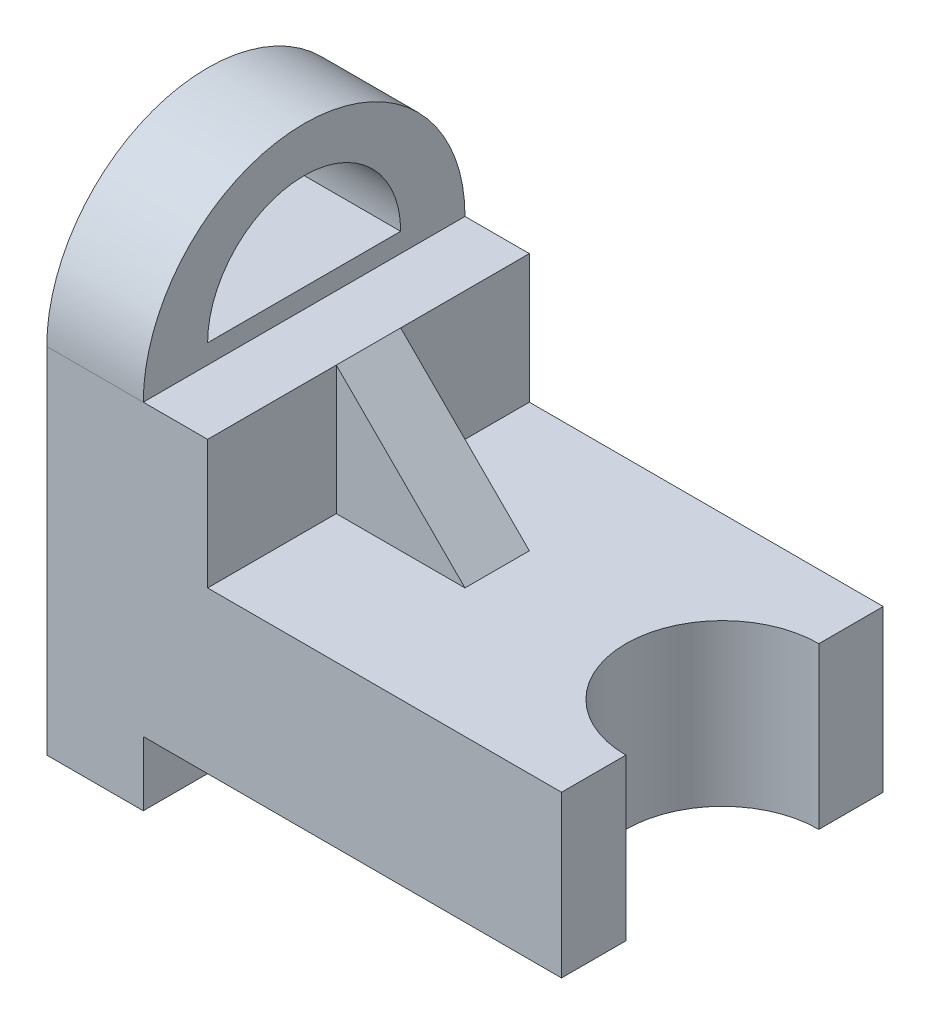
ISO-10303-21;
HEADER;
FILE_DESCRIPTION(('STEP AP214'),'2;1');
FILE_NAME('part.step','',(''),(''),'','','');
FILE_SCHEMA(('AUTOMOTIVE_DESIGN { 1 0 10303 214 1 1 1 1 }'));
ENDSEC;
DATA;
#1=APPLICATION_CONTEXT('core data for automotive mechanical design processes');
#2=APPLICATION_PROTOCOL_DEFINITION('international standard','automotive_design',2000,#1);
#3=PRODUCT_CONTEXT('',#1,'mechanical');
#4=PRODUCT('Part','Part','',(#3));
#5=PRODUCT_RELATED_PRODUCT_CATEGORY('part','',(#4));
#6=PRODUCT_DEFINITION_FORMATION('','',#4);
#7=PRODUCT_DEFINITION_CONTEXT('part definition',#1,'design');
#8=PRODUCT_DEFINITION('design','',#6,#7);
#9=PRODUCT_DEFINITION_SHAPE('','',#8);
#10=(LENGTH_UNIT() NAMED_UNIT(*) SI_UNIT(.MILLI.,.METRE.));
#11=(NAMED_UNIT(*) PLANE_ANGLE_UNIT() SI_UNIT($,.RADIAN.));
#12=(NAMED_UNIT(*) SI_UNIT($,.STERADIAN.) SOLID_ANGLE_UNIT());
#13=UNCERTAINTY_MEASURE_WITH_UNIT(LENGTH_MEASURE(1.E-05),#10,'distance_accuracy_value','');
#14=(GEOMETRIC_REPRESENTATION_CONTEXT(3) GLOBAL_UNCERTAINTY_ASSIGNED_CONTEXT((#13)) GLOBAL_UNIT_ASSIGNED_CONTEXT((#10,
#11,#12)) REPRESENTATION_CONTEXT('',''));
#15=CARTESIAN_POINT('',(0.,0.,0.));
#16=DIRECTION('',(0.,0.,1.));
#17=DIRECTION('',(1.,0.,0.));
#18=AXIS2_PLACEMENT_3D('',#15,#16,#17);
#19=CARTESIAN_POINT('',(40.,35.,20.));
#20=DIRECTION('',(0.707106781186547,0.707106781186548,0.));
#21=DIRECTION('',(-0.707106781186548,0.707106781186547,0.));
#22=AXIS2_PLACEMENT_3D('',#19,#20,#21);
#23=PLANE('',#22);
#24=DIRECTION('',(0.,0.,1.));
#25=VECTOR('',#24,1.);
#26=CARTESIAN_POINT('',(20.,55.,20.));
#27=LINE('',#26,#25);
#28=CARTESIAN_POINT('',(20.,55.,20.));
#29=VERTEX_POINT('',#28);
#30=CARTESIAN_POINT('',(20.,55.,30.));
#31=VERTEX_POINT('',#30);
#32=EDGE_CURVE('E179',#29,#31,#27,.T.);
#33=ORIENTED_EDGE('',*,*,#32,.T.);
#34=DIRECTION('',(-0.707106781186548,0.707106781186547,0.));
#35=VECTOR('',#34,1.);
#36=CARTESIAN_POINT('',(40.,35.,30.));
#37=LINE('',#36,#35);
#38=CARTESIAN_POINT('',(40.,35.,30.));
#39=VERTEX_POINT('',#38);
#40=EDGE_CURVE('E166',#39,#31,#37,.T.);
#41=ORIENTED_EDGE('',*,*,#40,.F.);
#42=DIRECTION('',(0.,0.,1.));
#43=VECTOR('',#42,1.);
#44=CARTESIAN_POINT('',(40.,35.,20.));
#45=LINE('',#44,#43);
#46=CARTESIAN_POINT('',(40.,35.,20.));
#47=VERTEX_POINT('',#46);
#48=EDGE_CURVE('E189',#47,#39,#45,.T.);
#49=ORIENTED_EDGE('',*,*,#48,.F.);
#50=DIRECTION('',(-0.707106781186548,0.707106781186547,0.));
#51=VECTOR('',#50,1.);
#52=CARTESIAN_POINT('',(40.,35.,20.));
#53=LINE('',#52,#51);
#54=EDGE_CURVE('E190',#47,#29,#53,.T.);
#55=ORIENTED_EDGE('',*,*,#54,.T.);
#56=EDGE_LOOP('',(#33,#41,#49,#55));
#57=FACE_BOUND('',#56,.T.);
#58=ADVANCED_FACE('F44',(#57),#23,.T.);
#59=CARTESIAN_POINT('',(20.,0.,0.));
#60=DIRECTION('',(-1.,0.,0.));
#61=DIRECTION('',(0.,0.,1.));
#62=AXIS2_PLACEMENT_3D('',#59,#60,#61);
#63=PLANE('',#62);
#64=DIRECTION('',(0.,-1.,0.));
#65=VECTOR('',#64,1.);
#66=CARTESIAN_POINT('',(20.,55.,20.));
#67=LINE('',#66,#65);
#68=CARTESIAN_POINT('',(20.,35.,20.));
#69=VERTEX_POINT('',#68);
#70=EDGE_CURVE('E195',#29,#69,#67,.T.);
#71=ORIENTED_EDGE('',*,*,#70,.T.);
#72=DIRECTION('',(0.,0.,-1.));
#73=VECTOR('',#72,1.);
#74=CARTESIAN_POINT('',(20.,35.,0.));
#75=LINE('',#74,#73);
#76=CARTESIAN_POINT('',(20.,35.,0.));
#77=VERTEX_POINT('',#76);
#78=EDGE_CURVE('E222',#69,#77,#75,.T.);
#79=ORIENTED_EDGE('',*,*,#78,.T.);
#80=DIRECTION('',(0.,1.,0.));
#81=VECTOR('',#80,1.);
#82=CARTESIAN_POINT('',(20.,55.,0.));
#83=LINE('',#82,#81);
#84=CARTESIAN_POINT('',(20.,55.,0.));
#85=VERTEX_POINT('',#84);
#86=EDGE_CURVE('E225',#77,#85,#83,.T.);
#87=ORIENTED_EDGE('',*,*,#86,.T.);
#88=DIRECTION('',(0.,0.,1.));
#89=VECTOR('',#88,1.);
#90=CARTESIAN_POINT('',(20.,55.,50.));
#91=LINE('',#90,#89);
#92=EDGE_CURVE('E223',#85,#29,#91,.T.);
#93=ORIENTED_EDGE('',*,*,#92,.T.);
#94=EDGE_LOOP('',(#71,#79,#87,#93));
#95=FACE_BOUND('',#94,.T.);
#96=ADVANCED_FACE('F328',(#95),#63,.F.);
#97=CARTESIAN_POINT('',(75.,35.,50.));
#98=DIRECTION('',(-1.,0.,0.));
#99=DIRECTION('',(0.,0.,1.));
#100=AXIS2_PLACEMENT_3D('',#97,#98,#99);
#101=PLANE('',#100);
#102=DIRECTION('',(0.,0.,-1.));
#103=VECTOR('',#102,1.);
#104=CARTESIAN_POINT('',(75.,10.,50.));
#105=LINE('',#104,#103);
#106=CARTESIAN_POINT('',(75.,10.,50.));
#107=VERTEX_POINT('',#106);
#108=CARTESIAN_POINT('',(75.,10.,40.));
#109=VERTEX_POINT('',#108);
#110=EDGE_CURVE('E278',#107,#109,#105,.T.);
#111=ORIENTED_EDGE('',*,*,#110,.T.);
#112=DIRECTION('',(0.,1.,0.));
#113=VECTOR('',#112,1.);
#114=CARTESIAN_POINT('',(75.,10.,40.));
#115=LINE('',#114,#113);
#116=CARTESIAN_POINT('',(75.,35.,40.));
#117=VERTEX_POINT('',#116);
#118=EDGE_CURVE('E196',#109,#117,#115,.T.);
#119=ORIENTED_EDGE('',*,*,#118,.T.);
#120=DIRECTION('',(0.,0.,-1.));
#121=VECTOR('',#120,1.);
#122=CARTESIAN_POINT('',(75.,35.,50.));
#123=LINE('',#122,#121);
#124=CARTESIAN_POINT('',(75.,35.,50.));
#125=VERTEX_POINT('',#124);
#126=EDGE_CURVE('E277',#125,#117,#123,.T.);
#127=ORIENTED_EDGE('',*,*,#126,.F.);
#128=DIRECTION('',(0.,1.,0.));
#129=VECTOR('',#128,1.);
#130=CARTESIAN_POINT('',(75.,35.,50.));
#131=LINE('',#130,#129);
#132=EDGE_CURVE('E251',#107,#125,#131,.T.);
#133=ORIENTED_EDGE('',*,*,#132,.F.);
#134=EDGE_LOOP('',(#111,#119,#127,#133));
#135=FACE_BOUND('',#134,.T.);
#136=ADVANCED_FACE('F304',(#135),#101,.F.);
#137=CARTESIAN_POINT('',(10.,35.,50.));
#138=DIRECTION('',(0.,-1.,0.));
#139=DIRECTION('',(0.,0.,-1.));
#140=AXIS2_PLACEMENT_3D('',#137,#138,#139);
#141=PLANE('',#140);
#142=DIRECTION('',(1.,0.,0.));
#143=VECTOR('',#142,1.);
#144=CARTESIAN_POINT('',(20.,35.,20.));
#145=LINE('',#144,#143);
#146=EDGE_CURVE('E66',#69,#47,#145,.T.);
#147=ORIENTED_EDGE('',*,*,#146,.T.);
#148=ORIENTED_EDGE('',*,*,#48,.T.);
#149=DIRECTION('',(1.,0.,0.));
#150=VECTOR('',#149,1.);
#151=CARTESIAN_POINT('',(20.,35.,30.));
#152=LINE('',#151,#150);
#153=CARTESIAN_POINT('',(20.,35.,30.));
#154=VERTEX_POINT('',#153);
#155=EDGE_CURVE('E58',#154,#39,#152,.T.);
#156=ORIENTED_EDGE('',*,*,#155,.F.);
#157=DIRECTION('',(0.,0.,1.));
#158=VECTOR('',#157,1.);
#159=CARTESIAN_POINT('',(20.,35.,30.));
#160=LINE('',#159,#158);
#161=CARTESIAN_POINT('',(20.,35.,50.));
#162=VERTEX_POINT('',#161);
#163=EDGE_CURVE('E170',#154,#162,#160,.T.);
#164=ORIENTED_EDGE('',*,*,#163,.T.);
#165=DIRECTION('',(-1.,0.,0.));
#166=VECTOR('',#165,1.);
#167=CARTESIAN_POINT('',(10.,35.,50.));
#168=LINE('',#167,#166);
#169=EDGE_CURVE('E257',#125,#162,#168,.T.);
#170=ORIENTED_EDGE('',*,*,#169,.F.);
#171=ORIENTED_EDGE('',*,*,#126,.T.);
#172=CARTESIAN_POINT('',(75.,35.,25.));
#173=DIRECTION('',(0.,1.,0.));
#174=DIRECTION('',(0.,0.,1.));
#175=AXIS2_PLACEMENT_3D('',#172,#173,#174);
#176=CIRCLE('',#175,15.);
#177=CARTESIAN_POINT('',(75.,35.,9.99999999999999));
#178=VERTEX_POINT('',#177);
#179=EDGE_CURVE('E188',#178,#117,#176,.T.);
#180=ORIENTED_EDGE('',*,*,#179,.F.);
#181=CARTESIAN_POINT('',(75.,35.,0.));
#182=VERTEX_POINT('',#181);
#183=EDGE_CURVE('E263',#178,#182,#123,.T.);
#184=ORIENTED_EDGE('',*,*,#183,.T.);
#185=DIRECTION('',(-1.,0.,0.));
#186=VECTOR('',#185,1.);
#187=CARTESIAN_POINT('',(10.,35.,0.));
#188=LINE('',#187,#186);
#189=EDGE_CURVE('E272',#182,#77,#188,.T.);
#190=ORIENTED_EDGE('',*,*,#189,.T.);
#191=ORIENTED_EDGE('',*,*,#78,.F.);
#192=EDGE_LOOP('',(#147,#148,#156,#164,#170,#171,#180,#184,#190,#191));
#193=FACE_BOUND('',#192,.T.);
#194=ADVANCED_FACE('F326',(#193),#141,.F.);
#195=CARTESIAN_POINT('',(10.,55.,50.));
#196=DIRECTION('',(-1.,0.,0.));
#197=DIRECTION('',(0.,0.,1.));
#198=AXIS2_PLACEMENT_3D('',#195,#196,#197);
#199=PLANE('',#198);
#200=CARTESIAN_POINT('',(10.,58.,25.));
#201=DIRECTION('',(1.,0.,0.));
#202=DIRECTION('',(0.,0.,-1.));
#203=AXIS2_PLACEMENT_3D('',#200,#201,#202);
#204=CIRCLE('',#203,15.);
#205=CARTESIAN_POINT('',(10.,58.,10.));
#206=VERTEX_POINT('',#205);
#207=CARTESIAN_POINT('',(10.,58.,40.));
#208=VERTEX_POINT('',#207);
#209=EDGE_CURVE('E209',#206,#208,#204,.T.);
#210=ORIENTED_EDGE('',*,*,#209,.F.);
#211=DIRECTION('',(0.,0.,-1.));
#212=VECTOR('',#211,1.);
#213=CARTESIAN_POINT('',(10.,58.,0.));
#214=LINE('',#213,#212);
#215=EDGE_CURVE('E204',#208,#206,#214,.T.);
#216=ORIENTED_EDGE('',*,*,#215,.F.);
#217=EDGE_LOOP('',(#210,#216));
#218=FACE_BOUND('',#217,.T.);
#219=DIRECTION('',(0.,0.,1.));
#220=VECTOR('',#219,1.);
#221=CARTESIAN_POINT('',(10.,55.,50.));
#222=LINE('',#221,#220);
#223=CARTESIAN_POINT('',(10.,55.,0.));
#224=VERTEX_POINT('',#223);
#225=CARTESIAN_POINT('',(10.,55.,50.));
#226=VERTEX_POINT('',#225);
#227=EDGE_CURVE('E216',#224,#226,#222,.T.);
#228=ORIENTED_EDGE('',*,*,#227,.F.);
#229=CARTESIAN_POINT('',(10.,55.,25.));
#230=DIRECTION('',(-1.,0.,0.));
#231=DIRECTION('',(0.,0.,1.));
#232=AXIS2_PLACEMENT_3D('',#229,#230,#231);
#233=CIRCLE('',#232,25.);
#234=EDGE_CURVE('E231',#226,#224,#233,.T.);
#235=ORIENTED_EDGE('',*,*,#234,.F.);
#236=EDGE_LOOP('',(#228,#235));
#237=FACE_BOUND('',#236,.T.);
#238=ADVANCED_FACE('F321',(#218,#237),#199,.F.);
#239=CARTESIAN_POINT('',(10.,0.,50.));
#240=DIRECTION('',(0.,1.,0.));
#241=DIRECTION('',(0.,0.,1.));
#242=AXIS2_PLACEMENT_3D('',#239,#240,#241);
#243=PLANE('',#242);
#244=DIRECTION('',(1.,0.,0.));
#245=VECTOR('',#244,1.);
#246=CARTESIAN_POINT('',(10.,0.,50.));
#247=LINE('',#246,#245);
#248=CARTESIAN_POINT('',(-5.,0.,50.));
#249=VERTEX_POINT('',#248);
#250=CARTESIAN_POINT('',(10.,0.,50.));
#251=VERTEX_POINT('',#250);
#252=EDGE_CURVE('E250',#249,#251,#247,.T.);
#253=ORIENTED_EDGE('',*,*,#252,.F.);
#254=DIRECTION('',(0.,0.,1.));
#255=VECTOR('',#254,1.);
#256=CARTESIAN_POINT('',(-5.,0.,50.));
#257=LINE('',#256,#255);
#258=CARTESIAN_POINT('',(-5.,0.,0.));
#259=VERTEX_POINT('',#258);
#260=EDGE_CURVE('E239',#259,#249,#257,.T.);
#261=ORIENTED_EDGE('',*,*,#260,.F.);
#262=DIRECTION('',(1.,0.,0.));
#263=VECTOR('',#262,1.);
#264=CARTESIAN_POINT('',(10.,0.,0.));
#265=LINE('',#264,#263);
#266=CARTESIAN_POINT('',(10.,0.,0.));
#267=VERTEX_POINT('',#266);
#268=EDGE_CURVE('E246',#259,#267,#265,.T.);
#269=ORIENTED_EDGE('',*,*,#268,.T.);
#270=DIRECTION('',(0.,0.,-1.));
#271=VECTOR('',#270,1.);
#272=CARTESIAN_POINT('',(10.,0.,50.));
#273=LINE('',#272,#271);
#274=EDGE_CURVE('E11',#251,#267,#273,.T.);
#275=ORIENTED_EDGE('',*,*,#274,.F.);
#276=EDGE_LOOP('',(#253,#261,#269,#275));
#277=FACE_BOUND('',#276,.T.);
#278=ADVANCED_FACE('F50',(#277),#243,.F.);
#279=CARTESIAN_POINT('',(10.,10.,50.));
#280=DIRECTION('',(-1.,0.,0.));
#281=DIRECTION('',(0.,0.,1.));
#282=AXIS2_PLACEMENT_3D('',#279,#280,#281);
#283=PLANE('',#282);
#284=DIRECTION('',(0.,1.,0.));
#285=VECTOR('',#284,1.);
#286=CARTESIAN_POINT('',(10.,10.,0.));
#287=LINE('',#286,#285);
#288=CARTESIAN_POINT('',(10.,10.,0.));
#289=VERTEX_POINT('',#288);
#290=EDGE_CURVE('E261',#267,#289,#287,.T.);
#291=ORIENTED_EDGE('',*,*,#290,.T.);
#292=DIRECTION('',(0.,0.,-1.));
#293=VECTOR('',#292,1.);
#294=CARTESIAN_POINT('',(10.,10.,50.));
#295=LINE('',#294,#293);
#296=CARTESIAN_POINT('',(10.,10.,50.));
#297=VERTEX_POINT('',#296);
#298=EDGE_CURVE('E52',#297,#289,#295,.T.);
#299=ORIENTED_EDGE('',*,*,#298,.F.);
#300=DIRECTION('',(0.,1.,0.));
#301=VECTOR('',#300,1.);
#302=CARTESIAN_POINT('',(10.,10.,50.));
#303=LINE('',#302,#301);
#304=EDGE_CURVE('E248',#251,#297,#303,.T.);
#305=ORIENTED_EDGE('',*,*,#304,.F.);
#306=ORIENTED_EDGE('',*,*,#274,.T.);
#307=EDGE_LOOP('',(#291,#299,#305,#306));
#308=FACE_BOUND('',#307,.T.);
#309=ADVANCED_FACE('F315',(#308),#283,.F.);
#310=CARTESIAN_POINT('',(75.,10.,50.));
#311=DIRECTION('',(0.,1.,0.));
#312=DIRECTION('',(0.,0.,1.));
#313=AXIS2_PLACEMENT_3D('',#310,#311,#312);
#314=PLANE('',#313);
#315=CARTESIAN_POINT('',(75.,10.,9.99999999999999));
#316=VERTEX_POINT('',#315);
#317=CARTESIAN_POINT('',(75.,10.,0.));
#318=VERTEX_POINT('',#317);
#319=EDGE_CURVE('E276',#316,#318,#105,.T.);
#320=ORIENTED_EDGE('',*,*,#319,.F.);
#321=CARTESIAN_POINT('',(75.,10.,25.));
#322=DIRECTION('',(0.,1.,0.));
#323=DIRECTION('',(0.,0.,1.));
#324=AXIS2_PLACEMENT_3D('',#321,#322,#323);
#325=CIRCLE('',#324,15.);
#326=EDGE_CURVE('E193',#316,#109,#325,.T.);
#327=ORIENTED_EDGE('',*,*,#326,.T.);
#328=ORIENTED_EDGE('',*,*,#110,.F.);
#329=DIRECTION('',(1.,0.,0.));
#330=VECTOR('',#329,1.);
#331=CARTESIAN_POINT('',(75.,10.,50.));
#332=LINE('',#331,#330);
#333=EDGE_CURVE('E255',#297,#107,#332,.T.);
#334=ORIENTED_EDGE('',*,*,#333,.F.);
#335=ORIENTED_EDGE('',*,*,#298,.T.);
#336=DIRECTION('',(1.,0.,0.));
#337=VECTOR('',#336,1.);
#338=CARTESIAN_POINT('',(75.,10.,0.));
#339=LINE('',#338,#337);
#340=EDGE_CURVE('E262',#289,#318,#339,.T.);
#341=ORIENTED_EDGE('',*,*,#340,.T.);
#342=EDGE_LOOP('',(#320,#327,#328,#334,#335,#341));
#343=FACE_BOUND('',#342,.T.);
#344=ADVANCED_FACE('F290',(#343),#314,.F.);
#345=ORIENTED_EDGE('',*,*,#183,.F.);
#346=DIRECTION('',(0.,1.,0.));
#347=VECTOR('',#346,1.);
#348=CARTESIAN_POINT('',(75.,10.,9.99999999999999));
#349=LINE('',#348,#347);
#350=EDGE_CURVE('E197',#316,#178,#349,.T.);
#351=ORIENTED_EDGE('',*,*,#350,.F.);
#352=ORIENTED_EDGE('',*,*,#319,.T.);
#353=DIRECTION('',(0.,1.,0.));
#354=VECTOR('',#353,1.);
#355=CARTESIAN_POINT('',(75.,35.,0.));
#356=LINE('',#355,#354);
#357=EDGE_CURVE('E270',#318,#182,#356,.T.);
#358=ORIENTED_EDGE('',*,*,#357,.T.);
#359=EDGE_LOOP('',(#345,#351,#352,#358));
#360=FACE_BOUND('',#359,.T.);
#361=ADVANCED_FACE('F297',(#360),#101,.F.);
#362=CARTESIAN_POINT('',(0.,0.,50.));
#363=DIRECTION('',(0.,0.,-1.));
#364=DIRECTION('',(-1.,0.,0.));
#365=AXIS2_PLACEMENT_3D('',#362,#363,#364);
#366=PLANE('',#365);
#367=ORIENTED_EDGE('',*,*,#169,.T.);
#368=DIRECTION('',(0.,-1.,0.));
#369=VECTOR('',#368,1.);
#370=CARTESIAN_POINT('',(20.,55.,50.));
#371=LINE('',#370,#369);
#372=CARTESIAN_POINT('',(20.,55.,50.));
#373=VERTEX_POINT('',#372);
#374=EDGE_CURVE('E173',#373,#162,#371,.T.);
#375=ORIENTED_EDGE('',*,*,#374,.F.);
#376=DIRECTION('',(-1.,0.,0.));
#377=VECTOR('',#376,1.);
#378=CARTESIAN_POINT('',(20.,55.,50.));
#379=LINE('',#378,#377);
#380=EDGE_CURVE('E182',#373,#226,#379,.T.);
#381=ORIENTED_EDGE('',*,*,#380,.T.);
#382=DIRECTION('',(-1.,0.,0.));
#383=VECTOR('',#382,1.);
#384=CARTESIAN_POINT('',(0.,55.,50.));
#385=LINE('',#384,#383);
#386=CARTESIAN_POINT('',(-5.,55.,50.));
#387=VERTEX_POINT('',#386);
#388=EDGE_CURVE('E259',#226,#387,#385,.T.);
#389=ORIENTED_EDGE('',*,*,#388,.T.);
#390=DIRECTION('',(0.,1.,0.));
#391=VECTOR('',#390,1.);
#392=CARTESIAN_POINT('',(-5.,55.,50.));
#393=LINE('',#392,#391);
#394=EDGE_CURVE('E243',#249,#387,#393,.T.);
#395=ORIENTED_EDGE('',*,*,#394,.F.);
#396=ORIENTED_EDGE('',*,*,#252,.T.);
#397=ORIENTED_EDGE('',*,*,#304,.T.);
#398=ORIENTED_EDGE('',*,*,#333,.T.);
#399=ORIENTED_EDGE('',*,*,#132,.T.);
#400=EDGE_LOOP('',(#367,#375,#381,#389,#395,#396,#397,#398,#399));
#401=FACE_BOUND('',#400,.T.);
#402=ADVANCED_FACE('F307',(#401),#366,.F.);
#403=CARTESIAN_POINT('',(0.,0.,0.));
#404=DIRECTION('',(0.,0.,-1.));
#405=DIRECTION('',(-1.,0.,0.));
#406=AXIS2_PLACEMENT_3D('',#403,#404,#405);
#407=PLANE('',#406);
#408=ORIENTED_EDGE('',*,*,#268,.F.);
#409=DIRECTION('',(0.,-1.,0.));
#410=VECTOR('',#409,1.);
#411=CARTESIAN_POINT('',(-5.,0.,0.));
#412=LINE('',#411,#410);
#413=CARTESIAN_POINT('',(-5.,55.,0.));
#414=VERTEX_POINT('',#413);
#415=EDGE_CURVE('E236',#414,#259,#412,.T.);
#416=ORIENTED_EDGE('',*,*,#415,.F.);
#417=DIRECTION('',(-1.,0.,0.));
#418=VECTOR('',#417,1.);
#419=CARTESIAN_POINT('',(0.,55.,0.));
#420=LINE('',#419,#418);
#421=EDGE_CURVE('E249',#224,#414,#420,.T.);
#422=ORIENTED_EDGE('',*,*,#421,.F.);
#423=DIRECTION('',(-1.,0.,0.));
#424=VECTOR('',#423,1.);
#425=CARTESIAN_POINT('',(20.,55.,0.));
#426=LINE('',#425,#424);
#427=EDGE_CURVE('E230',#85,#224,#426,.T.);
#428=ORIENTED_EDGE('',*,*,#427,.F.);
#429=ORIENTED_EDGE('',*,*,#86,.F.);
#430=ORIENTED_EDGE('',*,*,#189,.F.);
#431=ORIENTED_EDGE('',*,*,#357,.F.);
#432=ORIENTED_EDGE('',*,*,#340,.F.);
#433=ORIENTED_EDGE('',*,*,#290,.F.);
#434=EDGE_LOOP('',(#408,#416,#422,#428,#429,#430,#431,#432,#433));
#435=FACE_BOUND('',#434,.T.);
#436=ADVANCED_FACE('F294',(#435),#407,.T.);
#437=CARTESIAN_POINT('',(-5.,0.,0.));
#438=DIRECTION('',(1.,0.,0.));
#439=DIRECTION('',(0.,0.,-1.));
#440=AXIS2_PLACEMENT_3D('',#437,#438,#439);
#441=PLANE('',#440);
#442=CARTESIAN_POINT('',(-5.,58.,25.));
#443=DIRECTION('',(1.,0.,0.));
#444=DIRECTION('',(0.,0.,-1.));
#445=AXIS2_PLACEMENT_3D('',#442,#443,#444);
#446=CIRCLE('',#445,15.);
#447=CARTESIAN_POINT('',(-5.,58.,10.));
#448=VERTEX_POINT('',#447);
#449=CARTESIAN_POINT('',(-5.,58.,40.));
#450=VERTEX_POINT('',#449);
#451=EDGE_CURVE('E206',#448,#450,#446,.T.);
#452=ORIENTED_EDGE('',*,*,#451,.T.);
#453=DIRECTION('',(0.,0.,-1.));
#454=VECTOR('',#453,1.);
#455=CARTESIAN_POINT('',(-5.,58.,0.));
#456=LINE('',#455,#454);
#457=EDGE_CURVE('E203',#450,#448,#456,.T.);
#458=ORIENTED_EDGE('',*,*,#457,.T.);
#459=EDGE_LOOP('',(#452,#458));
#460=FACE_BOUND('',#459,.T.);
#461=ORIENTED_EDGE('',*,*,#415,.T.);
#462=ORIENTED_EDGE('',*,*,#260,.T.);
#463=ORIENTED_EDGE('',*,*,#394,.T.);
#464=CARTESIAN_POINT('',(-5.,55.,25.));
#465=DIRECTION('',(-1.,0.,0.));
#466=DIRECTION('',(0.,0.,1.));
#467=AXIS2_PLACEMENT_3D('',#464,#465,#466);
#468=CIRCLE('',#467,25.);
#469=EDGE_CURVE('E235',#387,#414,#468,.T.);
#470=ORIENTED_EDGE('',*,*,#469,.T.);
#471=EDGE_LOOP('',(#461,#462,#463,#470));
#472=FACE_BOUND('',#471,.T.);
#473=ADVANCED_FACE('F319',(#460,#472),#441,.F.);
#474=CARTESIAN_POINT('',(10.,55.,25.));
#475=DIRECTION('',(-1.,0.,0.));
#476=DIRECTION('',(0.,0.,1.));
#477=AXIS2_PLACEMENT_3D('',#474,#475,#476);
#478=CYLINDRICAL_SURFACE('',#477,25.);
#479=ORIENTED_EDGE('',*,*,#469,.F.);
#480=ORIENTED_EDGE('',*,*,#388,.F.);
#481=ORIENTED_EDGE('',*,*,#234,.T.);
#482=ORIENTED_EDGE('',*,*,#421,.T.);
#483=EDGE_LOOP('',(#479,#480,#481,#482));
#484=FACE_BOUND('',#483,.T.);
#485=ADVANCED_FACE('F318',(#484),#478,.T.);
#486=CARTESIAN_POINT('',(20.,55.,50.));
#487=DIRECTION('',(0.,-1.,0.));
#488=DIRECTION('',(0.,0.,-1.));
#489=AXIS2_PLACEMENT_3D('',#486,#487,#488);
#490=PLANE('',#489);
#491=ORIENTED_EDGE('',*,*,#227,.T.);
#492=ORIENTED_EDGE('',*,*,#380,.F.);
#493=DIRECTION('',(0.,0.,1.));
#494=VECTOR('',#493,1.);
#495=CARTESIAN_POINT('',(20.,55.,30.));
#496=LINE('',#495,#494);
#497=EDGE_CURVE('E165',#31,#373,#496,.T.);
#498=ORIENTED_EDGE('',*,*,#497,.F.);
#499=ORIENTED_EDGE('',*,*,#32,.F.);
#500=ORIENTED_EDGE('',*,*,#92,.F.);
#501=ORIENTED_EDGE('',*,*,#427,.T.);
#502=EDGE_LOOP('',(#491,#492,#498,#499,#500,#501));
#503=FACE_BOUND('',#502,.T.);
#504=ADVANCED_FACE('F178',(#503),#490,.F.);
#505=CARTESIAN_POINT('',(-5.,58.,0.));
#506=DIRECTION('',(0.,-1.,0.));
#507=DIRECTION('',(0.,0.,-1.));
#508=AXIS2_PLACEMENT_3D('',#505,#506,#507);
#509=PLANE('',#508);
#510=ORIENTED_EDGE('',*,*,#215,.T.);
#511=DIRECTION('',(1.,0.,0.));
#512=VECTOR('',#511,1.);
#513=CARTESIAN_POINT('',(-5.,58.,10.));
#514=LINE('',#513,#512);
#515=EDGE_CURVE('E215',#448,#206,#514,.T.);
#516=ORIENTED_EDGE('',*,*,#515,.F.);
#517=ORIENTED_EDGE('',*,*,#457,.F.);
#518=DIRECTION('',(1.,0.,0.));
#519=VECTOR('',#518,1.);
#520=CARTESIAN_POINT('',(-5.,58.,40.));
#521=LINE('',#520,#519);
#522=EDGE_CURVE('E218',#450,#208,#521,.T.);
#523=ORIENTED_EDGE('',*,*,#522,.T.);
#524=EDGE_LOOP('',(#510,#516,#517,#523));
#525=FACE_BOUND('',#524,.T.);
#526=ADVANCED_FACE('F342',(#525),#509,.F.);
#527=CARTESIAN_POINT('',(-5.,58.,25.));
#528=DIRECTION('',(1.,0.,0.));
#529=DIRECTION('',(0.,0.,-1.));
#530=AXIS2_PLACEMENT_3D('',#527,#528,#529);
#531=CYLINDRICAL_SURFACE('',#530,15.);
#532=ORIENTED_EDGE('',*,*,#209,.T.);
#533=ORIENTED_EDGE('',*,*,#522,.F.);
#534=ORIENTED_EDGE('',*,*,#451,.F.);
#535=ORIENTED_EDGE('',*,*,#515,.T.);
#536=EDGE_LOOP('',(#532,#533,#534,#535));
#537=FACE_BOUND('',#536,.T.);
#538=ADVANCED_FACE('F335',(#537),#531,.F.);
#539=CARTESIAN_POINT('',(75.,10.,25.));
#540=DIRECTION('',(0.,1.,0.));
#541=DIRECTION('',(0.,0.,1.));
#542=AXIS2_PLACEMENT_3D('',#539,#540,#541);
#543=CYLINDRICAL_SURFACE('',#542,15.);
#544=ORIENTED_EDGE('',*,*,#179,.T.);
#545=ORIENTED_EDGE('',*,*,#118,.F.);
#546=ORIENTED_EDGE('',*,*,#326,.F.);
#547=ORIENTED_EDGE('',*,*,#350,.T.);
#548=EDGE_LOOP('',(#544,#545,#546,#547));
#549=FACE_BOUND('',#548,.T.);
#550=ADVANCED_FACE('F327',(#549),#543,.F.);
#551=CARTESIAN_POINT('',(0.,0.,20.));
#552=DIRECTION('',(0.,0.,1.));
#553=DIRECTION('',(1.,0.,0.));
#554=AXIS2_PLACEMENT_3D('',#551,#552,#553);
#555=PLANE('',#554);
#556=ORIENTED_EDGE('',*,*,#54,.F.);
#557=ORIENTED_EDGE('',*,*,#146,.F.);
#558=ORIENTED_EDGE('',*,*,#70,.F.);
#559=EDGE_LOOP('',(#556,#557,#558));
#560=FACE_BOUND('',#559,.T.);
#561=ADVANCED_FACE('F334',(#560),#555,.F.);
#562=CARTESIAN_POINT('',(20.,55.,30.));
#563=DIRECTION('',(-1.,0.,0.));
#564=DIRECTION('',(0.,0.,1.));
#565=AXIS2_PLACEMENT_3D('',#562,#563,#564);
#566=PLANE('',#565);
#567=ORIENTED_EDGE('',*,*,#374,.T.);
#568=ORIENTED_EDGE('',*,*,#163,.F.);
#569=DIRECTION('',(0.,-1.,0.));
#570=VECTOR('',#569,1.);
#571=CARTESIAN_POINT('',(20.,55.,30.));
#572=LINE('',#571,#570);
#573=EDGE_CURVE('E158',#31,#154,#572,.T.);
#574=ORIENTED_EDGE('',*,*,#573,.F.);
#575=ORIENTED_EDGE('',*,*,#497,.T.);
#576=EDGE_LOOP('',(#567,#568,#574,#575));
#577=FACE_BOUND('',#576,.T.);
#578=ADVANCED_FACE('F162',(#577),#566,.F.);
#579=CARTESIAN_POINT('',(0.,0.,30.));
#580=DIRECTION('',(0.,0.,1.));
#581=DIRECTION('',(1.,0.,0.));
#582=AXIS2_PLACEMENT_3D('',#579,#580,#581);
#583=PLANE('',#582);
#584=ORIENTED_EDGE('',*,*,#40,.T.);
#585=ORIENTED_EDGE('',*,*,#573,.T.);
#586=ORIENTED_EDGE('',*,*,#155,.T.);
#587=EDGE_LOOP('',(#584,#585,#586));
#588=FACE_BOUND('',#587,.T.);
#589=ADVANCED_FACE('F167',(#588),#583,.T.);
#590=CLOSED_SHELL('',(#58,#96,#136,#194,#238,#278,#309,#344,#361,#402,#436,#473,#485,#504,#526,
#538,#550,#561,#578,#589));
#591=MANIFOLD_SOLID_BREP('B2',#590);
#592=ADVANCED_BREP_SHAPE_REPRESENTATION('',(#18,#591),#14);
#593=SHAPE_DEFINITION_REPRESENTATION(#9,#592);
ENDSEC;
END-ISO-10303-21;
